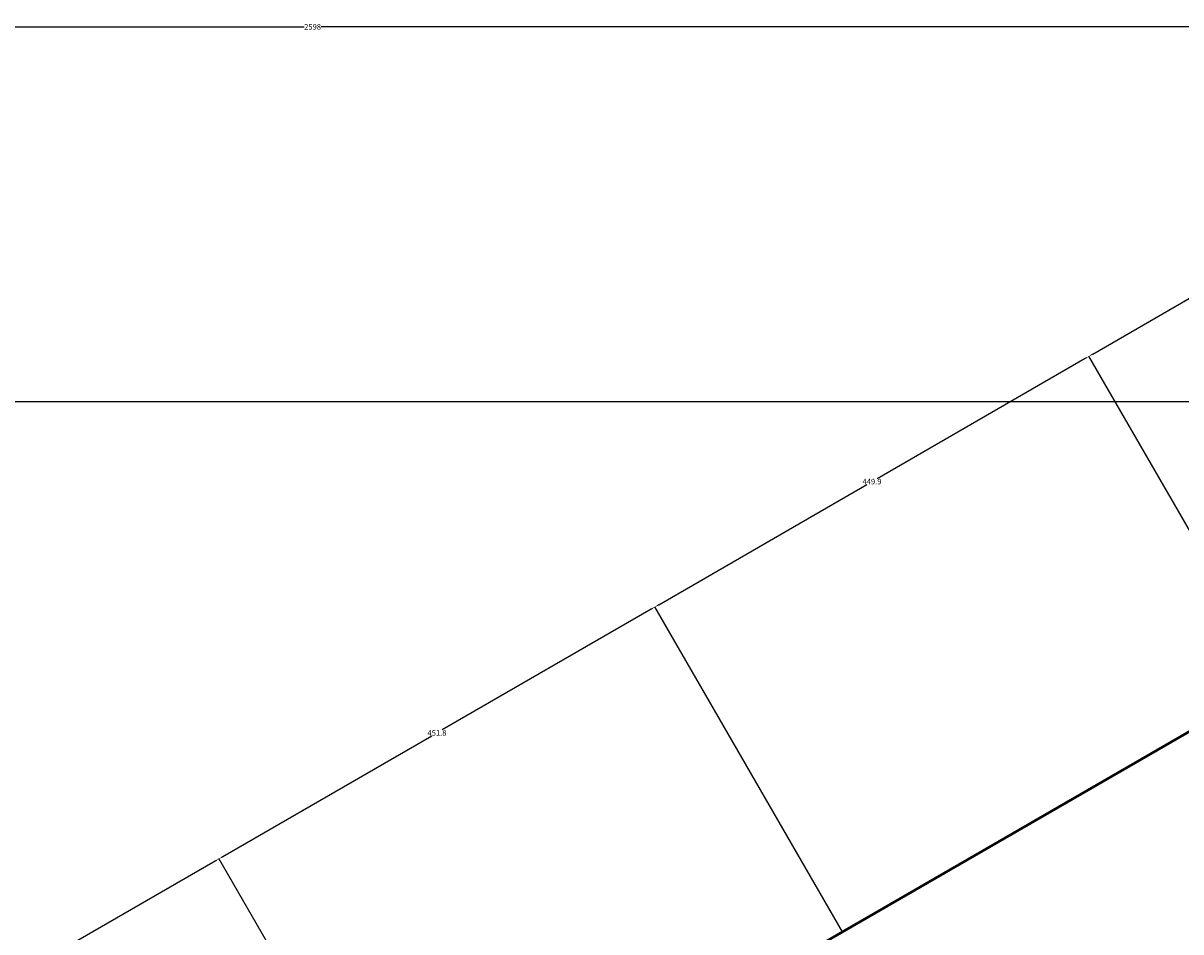
# Model space of a CAD drawing. Units: metres. Extents: x -2391 to 4922, y -635 to 4845.
# Tile 21 of 37: x -1008 to 31, y 4030 to 4845. Entities that reach past the tile are written whole.
import ezdxf

# ---------------------------------------------------------------- set-up
doc = ezdxf.new("R2010")
doc.units = ezdxf.units.M
doc.header["$MEASUREMENT"] = 0
doc.layers.add('A-ANNO-DIMS', color=2, linetype='Continuous', lineweight=18)
doc.layers.add('A-WALL', color=7, linetype='Continuous', lineweight=50)
doc.styles.get("Standard").update_dxf_attribs({"font": 'arial.ttf'})
doc.dimstyles.get("Standard").update_dxf_attribs({"dimtxt": 5, "dimasz": 4, "dimexe": 0.18, "dimexo": 0.0625, "dimgap": 0.09, "dimtad": 0, "dimtih": 1, "dimtoh": 1, "dimdec": 0, "dimzin": 0, "dimdsep": 46, "dimtxsty": 'Standard', "dimcen": 0.09, "dimadec": 0, "dimazin": 0, "dimtfac": 1, "dimtdec": 0, "dimtofl": 0, "dimtmove": 0, "dimatfit": 3, "dimfxl": 1, "dimtolj": 1, "dimtzin": 0, "dimarcsym": 0})

# ---------------------------------------------------------------- blocks, each defined once
blk = doc.blocks.new('*D9')
at = {"layer": 'A-ANNO-DIMS', "color": 0, "lineweight": -2, "transparency": 16777216}
for p, q in [((-2047.3, 3005.3), (-2047.3, 4842)), ((-2043.3, 4841.8), (-755.9, 4841.8)), ((546.7, 4841.8), (-740.7, 4841.8)), ((550.7, 4505.3), (550.7, 4842))]:
    blk.add_line(p, q, dxfattribs=at)
at = {"layer": 'A-ANNO-DIMS', "color": 0, "transparency": 16777216}
for points in [[(-2043.3, 4842.4), (-2043.3, 4841.1), (-2047.3, 4841.8)], [(546.7, 4842.4), (546.7, 4841.1), (550.7, 4841.8)]]:
    blk.add_solid(points, dxfattribs=at)
at = {"layer": 'Defpoints', "color": 0, "transparency": 16777216}
for p in [(550.7, 4841.8), (550.7, 4505.3), (-2047.3, 3005.3)]:
    blk.add_point(p, dxfattribs=at)
at = {"layer": 'A-ANNO-DIMS', "color": 0, "transparency": 16777216, "insert": (-748.3, 4841.8), "char_height": 5, "attachment_point": 5}
blk.add_mtext('\\A1;2598', dxfattribs=at)
blk = doc.blocks.new('*D10')
at = {"layer": 'A-ANNO-DIMS', "color": 0, "lineweight": -2, "transparency": 16777216}
for p, q in [((550.7, 4505.3), (-2384, 4505.3)), ((-2383.8, 4501.3), (-2383.8, 2107.9)), ((-2383.8, -290.7), (-2383.8, 2102.6)), ((-488.6, -294.7), (-2384, -294.7))]:
    blk.add_line(p, q, dxfattribs=at)
at = {"layer": 'A-ANNO-DIMS', "color": 0, "transparency": 16777216}
for points in [[(-2384.5, 4501.3), (-2383.2, 4501.3), (-2383.8, 4505.3)], [(-2384.5, -290.7), (-2383.2, -290.7), (-2383.8, -294.7)]]:
    blk.add_solid(points, dxfattribs=at)
at = {"layer": 'Defpoints', "color": 0, "transparency": 16777216}
for p in [(-2383.8, 4505.3), (550.7, 4505.3), (-488.5, -294.7)]:
    blk.add_point(p, dxfattribs=at)
at = {"layer": 'A-ANNO-DIMS', "color": 0, "transparency": 16777216, "insert": (-2383.8, 2105.3), "char_height": 5, "attachment_point": 5}
blk.add_mtext('\\A1;4800', dxfattribs=at)
blk = doc.blocks.new('*D37')
at = {"layer": 'A-ANNO-DIMS', "color": 0, "lineweight": -2, "transparency": 16777216}
for p, q in [((-664, 3804), (-832.3, 4095.5)), ((-835.7, 4093.4), (-1050.8, 3969.2)), ((-1275.1, 3839.7), (-1060, 3963.9)), ((-1110.4, 3546.3), (-1278.7, 3837.8))]:
    blk.add_line(p, q, dxfattribs=at)
at = {"layer": 'A-ANNO-DIMS', "color": 0, "transparency": 16777216}
for points in [[(-836, 4094), (-835.4, 4092.8), (-832.2, 4095.4)], [(-1275.5, 3840.2), (-1274.8, 3839.1), (-1278.6, 3837.7)]]:
    blk.add_solid(points, dxfattribs=at)
at = {"layer": 'Defpoints', "color": 0, "transparency": 16777216}
for p in [(-832.2, 4095.4), (-664, 3804), (-1110.4, 3546.2)]:
    blk.add_point(p, dxfattribs=at)
at = {"layer": 'A-ANNO-DIMS', "color": 0, "transparency": 16777216, "insert": (-1055.4, 3966.5), "char_height": 5, "attachment_point": 5}
blk.add_mtext('\\A1;515.4', dxfattribs=at)
blk = doc.blocks.new('*D38')
at = {"layer": 'A-ANNO-DIMS', "color": 0, "lineweight": -2, "transparency": 16777216}
for p, q in [((-444.4, 4319.3), (-632, 4211)), ((-272.7, 4029.9), (-441, 4321.4)), ((-828.8, 4097.4), (-641.2, 4205.7)), ((-664, 3804), (-832.3, 4095.5))]:
    blk.add_line(p, q, dxfattribs=at)
at = {"layer": 'A-ANNO-DIMS', "color": 0, "transparency": 16777216}
for points in [[(-444.8, 4319.9), (-444.1, 4318.7), (-441, 4321.3)], [(-829.1, 4098), (-828.4, 4096.8), (-832.2, 4095.4)]]:
    blk.add_solid(points, dxfattribs=at)
at = {"layer": 'Defpoints', "color": 0, "transparency": 16777216}
for p in [(-441, 4321.3), (-272.7, 4029.9), (-664, 3804)]:
    blk.add_point(p, dxfattribs=at)
at = {"layer": 'A-ANNO-DIMS', "color": 0, "transparency": 16777216, "insert": (-636.6, 4208.3), "char_height": 5, "attachment_point": 5}
blk.add_mtext('\\A1;451.8', dxfattribs=at)
blk = doc.blocks.new('*D39')
at = {"layer": 'A-ANNO-DIMS', "color": 0, "lineweight": -2, "transparency": 16777216}
for p, q in [((-54.8, 4544.2), (-241.6, 4436.4)), ((116.9, 4254.9), (-51.4, 4546.4)), ((-437.5, 4323.3), (-250.7, 4431.1)), ((-272.7, 4029.9), (-441, 4321.4))]:
    blk.add_line(p, q, dxfattribs=at)
at = {"layer": 'A-ANNO-DIMS', "color": 0, "transparency": 16777216}
for points in [[(-55.1, 4544.8), (-54.5, 4543.7), (-51.3, 4546.2)], [(-437.8, 4323.9), (-437.2, 4322.7), (-441, 4321.3)]]:
    blk.add_solid(points, dxfattribs=at)
at = {"layer": 'Defpoints', "color": 0, "transparency": 16777216}
for p in [(-51.3, 4546.2), (116.9, 4254.8), (-272.7, 4029.9)]:
    blk.add_point(p, dxfattribs=at)
at = {"layer": 'A-ANNO-DIMS', "color": 0, "transparency": 16777216, "insert": (-246.1, 4433.8), "char_height": 5, "attachment_point": 5}
blk.add_mtext('\\A1;449.9', dxfattribs=at)
blk = doc.blocks.new('*D40')
at = {"layer": 'A-ANNO-DIMS', "color": 0, "lineweight": -2, "transparency": 16777216}
for p, q in [((379, 4794.7), (170.2, 4674.1)), ((550.7, 4505.3), (382.4, 4796.8)), ((-47.9, 4548.2), (161, 4668.8)), ((116.9, 4254.9), (-51.4, 4546.4))]:
    blk.add_line(p, q, dxfattribs=at)
at = {"layer": 'A-ANNO-DIMS', "color": 0, "transparency": 16777216}
for points in [[(378.7, 4795.3), (379.4, 4794.1), (382.5, 4796.7)], [(-48.2, 4548.8), (-47.5, 4547.7), (-51.3, 4546.2)]]:
    blk.add_solid(points, dxfattribs=at)
at = {"layer": 'Defpoints', "color": 0, "transparency": 16777216}
for p in [(382.5, 4796.7), (550.7, 4505.3), (116.9, 4254.8)]:
    blk.add_point(p, dxfattribs=at)
at = {"layer": 'A-ANNO-DIMS', "color": 0, "transparency": 16777216, "insert": (165.6, 4671.5), "char_height": 5, "attachment_point": 5}
blk.add_mtext('\\A1;500.9', dxfattribs=at)

msp = doc.modelspace()

# ---------------------------------------------------------------- linework, layer by layer
at = {"layer": 'A-WALL'}
msp.add_line((-1008.1038, 3605.2763), (550.7419, 4505.2763), dxfattribs=at)

# ---------------------------------------------------------------- dimensions: what is measured, and where the dimension line sits
at = {"layer": 'A-ANNO-DIMS'}
dim = msp.add_linear_dim(base=(550.7419, 4841.7763), p1=(-2047.3343, 3005.2763), p2=(550.7419, 4505.2763), dimstyle='Standard', override={"dimdec": 0, "dimlfac": 1, "dimrnd": 0, "dimzin": 0, "dimdsep": 46, "dimlunit": 2}, dxfattribs=at)
dim.commit()
dim.dimension.update_dxf_attribs({"geometry": '*D9', "text_midpoint": (-748.2962, 4841.7763)})
for base, p1, p2, angle, override, picture, middle in [((382.4919, 4796.6938), (116.9223, 4254.8104), (550.7419, 4505.2763), 30, {"dimdec": 1, "dimlfac": 1, "dimrnd": 0, "dimzin": 0, "dimdsep": 46, "dimlunit": 2}, '*D40', (165.5821, 4671.4609)), ((-51.3277, 4546.228), (-272.7053, 4029.8588), (116.9223, 4254.8104), 30, {"dimdec": 1, "dimlfac": 1, "dimrnd": 0, "dimzin": 0, "dimdsep": 46, "dimlunit": 2}, '*D39', (-246.1415, 4433.7522)), ((-2383.8343, 4505.2763), (-488.4886, -294.7237), (550.7419, 4505.2763), 90, {"dimdec": 0, "dimlfac": 1, "dimrnd": 0, "dimzin": 0, "dimdsep": 46, "dimlunit": 2}, '*D10', (-2383.8343, 2105.2763)), ((-440.9553, 4321.2764), (-663.9742, 3803.9596), (-272.7053, 4029.8588), 30, {"dimdec": 1, "dimlfac": 1, "dimrnd": 0, "dimzin": 0, "dimdsep": 46, "dimlunit": 2}, '*D38', (-636.5898, 4208.3267)), ((-832.2242, 4095.3771), (-1110.3549, 3546.2416), (-663.9742, 3803.9596), 30, {"dimdec": 1, "dimlfac": 1, "dimrnd": 0, "dimzin": 0, "dimdsep": 46, "dimlunit": 2}, '*D37', (-1055.4146, 3966.5181))]:
    dim = msp.add_linear_dim(base=base, p1=p1, p2=p2, angle=angle, dimstyle='Standard', override=override, dxfattribs=at)
    dim.commit()
    dim.dimension.update_dxf_attribs({"geometry": picture, "text_midpoint": middle})

doc.saveas('drawing.dxf')
